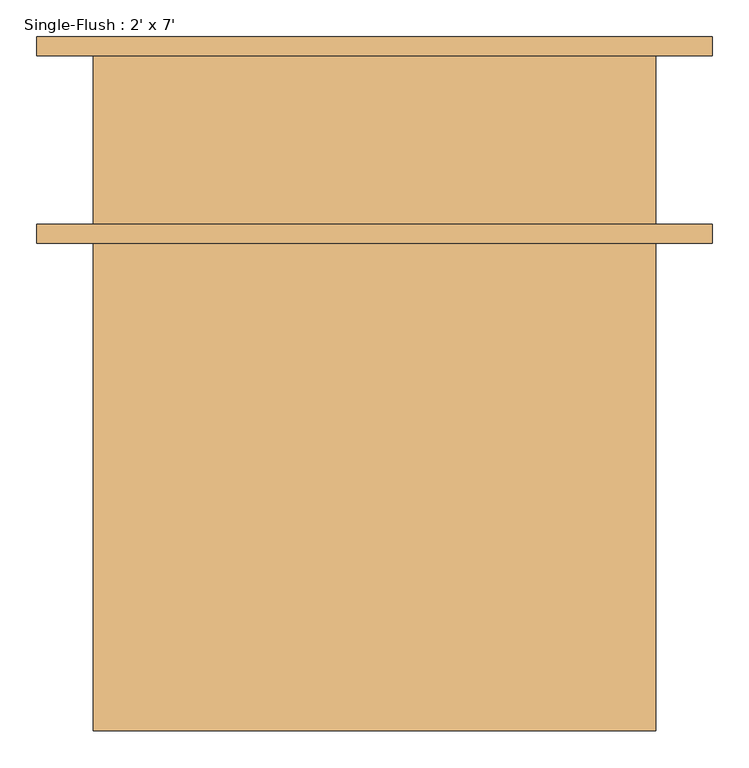
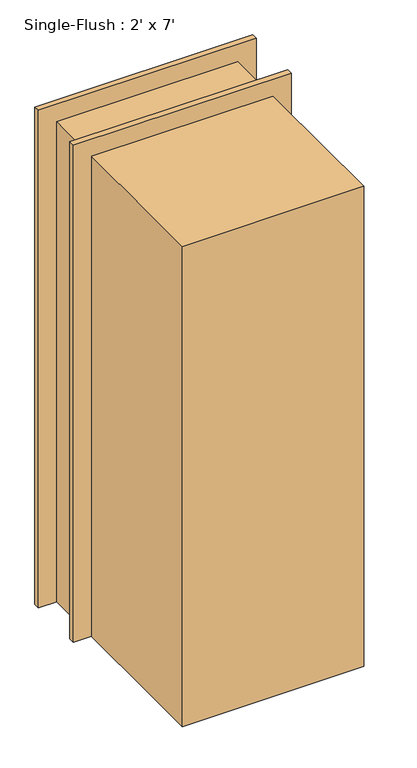
"""IFC4 building model written with IfcOpenShell, lengths in millimetres: door geometry, Single-Flush : 2' x 7'."""

from ifc_helpers import new_model, si_unit, frame, origin, origin_with_axes, place, context, project, spatial, polyline, outline, extrude, source, transform, mapped, element, save


def single_flush_2_x_7_f433b8c7(model_context):
    return source(origin(), model_context, "Body", "SweptSolid", [
        extrude(outline(polyline([(2209.8, -457.2), (0.0, -457.2), (0.0, -381.0), (2133.6, -381.0), (2133.6, 381.0), (0.0, 381.0), (0.0, 457.2), (2209.8, 457.2), (2209.8, -457.2)])), frame((0.0, 114.3, 0.0), z_axis=(0.0, 1.0, 0.0), x_axis=(0.0, 0.0, 1.0)), (0.0, 0.0, 1.0), 25.4),
        extrude(outline(polyline([(2209.8, 457.2), (2209.8, -457.2), (0.0, -457.2), (0.0, -381.0), (2133.6, -381.0), (2133.6, 381.0), (0.0, 381.0), (0.0, 457.2), (2209.8, 457.2)])), frame((0.0, -139.7, 0.0), z_axis=(0.0, 1.0, 0.0), x_axis=(0.0, 0.0, 1.0)), (0.0, 0.0, 1.0), 25.4),
        extrude(outline(polyline([(381.0, -800.1), (-381.0, -800.1), (-381.0, 114.3), (381.0, 114.3), (381.0, -800.1)])), origin_with_axes(), (0.0, 0.0, 1.0), 2133.6),
    ])


if __name__ == "__main__":
    model = new_model("IFC4")
    model_context = context("Model", 3, world=origin())
    ifc_project = project(units=[si_unit("LENGTHUNIT", "METRE", prefix="MILLI")], contexts=[model_context])
    site = spatial("IfcSite", under=ifc_project)
    building = spatial("IfcBuilding", under=site)
    placement = place(None, origin())
    single_flush_2_x_7_shape = single_flush_2_x_7_f433b8c7(model_context)
    element("IfcDoor", 1, ObjectType="Single-Flush : 2' x 7'", at=placement, inside=building, context=model_context, shape_type="MappedRepresentation", body=[
        mapped(single_flush_2_x_7_shape, transform((0.0, 0.0, 0.0), x_axis=(1.0, 0.0, 0.0), y_axis=(0.0, 1.0, 0.0), z_axis=(0.0, 0.0, 1.0))),
    ])
    save(model, "model.ifc")

# Revit data of these elements
# Type "Single-Flush : 2' x 7'"
#   Type Mark = "10"
#   Construction Type Id = "MDOOR"
#   Assembly Code = "C1020"
#   Analytic Construction = "Metal"
#   Thickness = 3' - 0"
#   Heat Transfer Coefficient (U) = 0.651978 BTU/(h·ft²·°F)
#   Height = 7' - 0"
#   Trim Projection Ext = 0' - 1"
#   Trim Projection Int = 0' - 1"
#   Trim Width = 0' - 3"
#   Width = 2' - 6"
#   Define Thermal Properties by = 1
#   Door Material = Door - Panel
#   Frame Material = Door - Frame
#   Visual Light Transmittance = 0
#   Solar Heat Gain Coefficient = 0
#   Function = (empty or 0)
#   Wall Closure = (empty or 0)
# Element 1 (IfcDoor, "Single-Flush : 2' x 7'")
#   Materials on its faces: "Door - Frame", "Door - Panel"
# Materials
#   "Door - Panel": class "Wood", colour RGB 210 159 95, transparency 0, Cost = 0
#   "Door - Frame": colour RGB 118 70 51, transparency 0, Cost = 0
